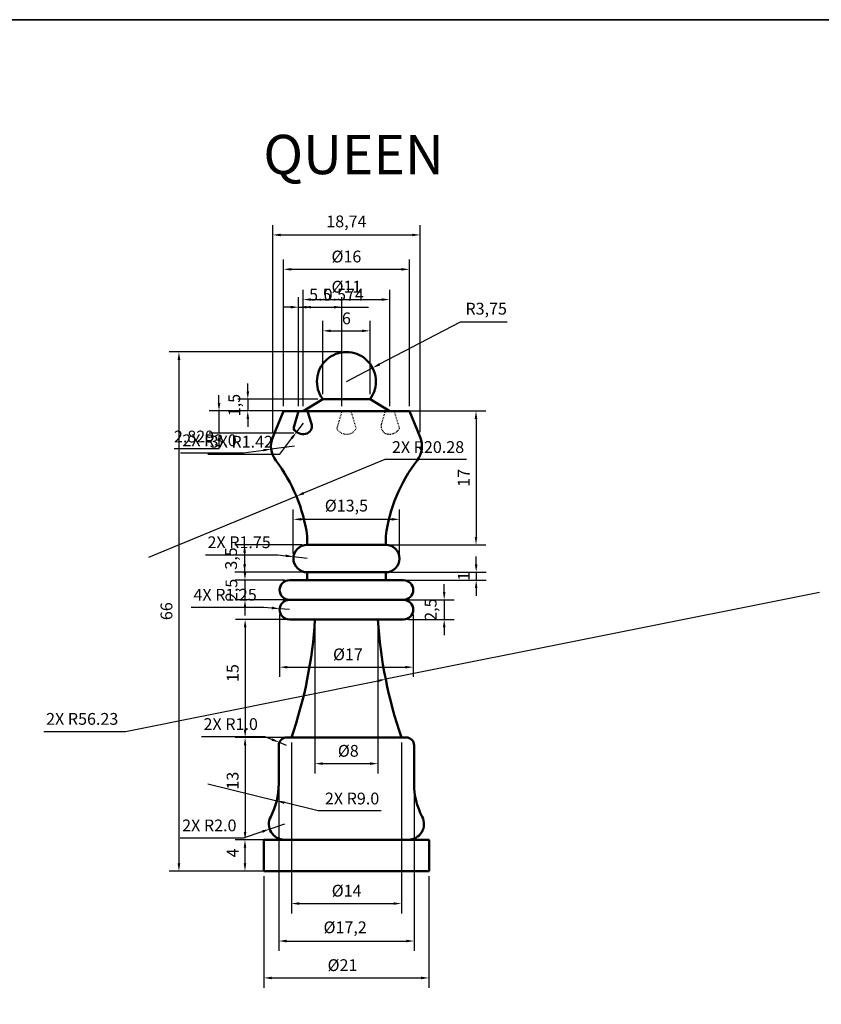
# Model space of a CAD drawing. Units: millimetres. Extents: x 172 to 469, y -14 to 196.
# Tile 4 of 5: x 279 to 381, y 71 to 196. Entities that reach past the tile are written whole.
import ezdxf

# ---------------------------------------------------------------- set-up
doc = ezdxf.new("R2010")
doc.units = ezdxf.units.MM
doc.header["$LTSCALE"] = 0.1
doc.linetypes.add('HIDDEN', pattern=[9.525, 6.35, -3.175])
for name, color, linetype, lineweight in [('M-DIMS', 2, 'Continuous', 25), ('M-HIDN', 1, 'HIDDEN', 25), ('M-OUTL', 7, 'Continuous', 50), ('M-TEXT', 3, 'Continuous', 25), ('M-TTLB', 7, 'Continuous', 35)]:
    doc.layers.add(name, color=color, linetype=linetype, lineweight=lineweight)
doc.styles.get("Standard").update_dxf_attribs({"font": 'arial.ttf'})
doc.dimstyles.new('ISO-25', dxfattribs={"dimtxt": 1.5, "dimasz": 1, "dimexe": 1.25, "dimexo": 0.625, "dimtad": 1, "dimtoh": 1, "dimtxsty": 'Standard', "dimcen": 2.5, "dimadec": 0, "dimazin": 0, "dimtfac": 1, "dimtmove": 0, "dimatfit": 3, "dimfxl": 1, "dimarcsym": 0})

# ---------------------------------------------------------------- blocks, each defined once
blk = doc.blocks.new('*D15')
at = {"layer": 'Defpoints', "color": 0, "ltscale": 0.1, "transparency": 16777216}
for p in [(328.72, 164.14), (312.72, 146.13), (328.72, 146.13)]:
    blk.add_point(p, dxfattribs=at)
at = {"layer": 'M-DIMS', "color": 0, "lineweight": -2, "ltscale": 0.1, "transparency": 16777216}
for p, q in [((312.72, 146.75), (312.72, 165.39)), ((328.72, 146.75), (328.72, 165.39)), ((313.72, 164.14), (327.72, 164.14))]:
    blk.add_line(p, q, dxfattribs=at)
at = {"layer": 'M-DIMS', "color": 0, "ltscale": 0.1, "transparency": 16777216}
for points in [[(313.72, 164.3), (313.72, 163.97), (312.72, 164.14)], [(327.72, 164.3), (327.72, 163.97), (328.72, 164.14)]]:
    blk.add_solid(points, dxfattribs=at)
at = {"layer": 'M-DIMS', "color": 0, "ltscale": 0.1, "transparency": 16777216, "insert": (320.72, 165.57), "char_height": 1.5, "attachment_point": 5}
blk.add_mtext('%%C16', dxfattribs=at)
blk = doc.blocks.new('*D16')
at = {"layer": 'Defpoints', "color": 0, "ltscale": 0.1, "transparency": 16777216}
for p in [(330.1, 168.51), (311.35, 142.82), (330.1, 142.82)]:
    blk.add_point(p, dxfattribs=at)
at = {"layer": 'M-DIMS', "color": 0, "lineweight": -2, "ltscale": 0.1, "transparency": 16777216}
for p, q in [((311.35, 143.44), (311.35, 169.76)), ((330.1, 143.44), (330.1, 169.76)), ((312.35, 168.51), (329.1, 168.51))]:
    blk.add_line(p, q, dxfattribs=at)
at = {"layer": 'M-DIMS', "color": 0, "ltscale": 0.1, "transparency": 16777216}
for points in [[(312.35, 168.67), (312.35, 168.34), (311.35, 168.51)], [(329.1, 168.67), (329.1, 168.34), (330.1, 168.51)]]:
    blk.add_solid(points, dxfattribs=at)
at = {"layer": 'M-DIMS', "color": 0, "ltscale": 0.1, "transparency": 16777216, "insert": (320.72, 170.03), "char_height": 1.5, "attachment_point": 5}
blk.add_mtext('18,74', dxfattribs=at)
blk = doc.blocks.new('*D17')
at = {"layer": 'Defpoints', "color": 0, "ltscale": 0.1, "transparency": 16777216}
for p in [(326.22, 160.29), (315.22, 146.13), (326.22, 146.13)]:
    blk.add_point(p, dxfattribs=at)
at = {"layer": 'M-DIMS', "color": 0, "lineweight": -2, "ltscale": 0.1, "transparency": 16777216}
for p, q in [((315.22, 146.75), (315.22, 161.54)), ((326.22, 146.75), (326.22, 161.54)), ((316.22, 160.29), (325.22, 160.29))]:
    blk.add_line(p, q, dxfattribs=at)
at = {"layer": 'M-DIMS', "color": 0, "ltscale": 0.1, "transparency": 16777216}
for points in [[(316.22, 160.46), (316.22, 160.13), (315.22, 160.29)], [(325.22, 160.46), (325.22, 160.13), (326.22, 160.29)]]:
    blk.add_solid(points, dxfattribs=at)
at = {"layer": 'M-DIMS', "color": 0, "ltscale": 0.1, "transparency": 16777216, "insert": (320.72, 161.73), "char_height": 1.5, "attachment_point": 5}
blk.add_mtext('%%C11', dxfattribs=at)
blk = doc.blocks.new('*D18')
at = {"layer": 'Defpoints', "color": 0, "ltscale": 0.1, "transparency": 16777216}
for p in [(323.72, 156.32), (317.72, 147.63), (323.72, 147.63)]:
    blk.add_point(p, dxfattribs=at)
at = {"layer": 'M-DIMS', "color": 0, "lineweight": -2, "ltscale": 0.1, "transparency": 16777216}
for p, q in [((317.72, 148.25), (317.72, 157.57)), ((323.72, 148.25), (323.72, 157.57)), ((318.72, 156.32), (322.72, 156.32))]:
    blk.add_line(p, q, dxfattribs=at)
at = {"layer": 'M-DIMS', "color": 0, "ltscale": 0.1, "transparency": 16777216}
for points in [[(318.72, 156.48), (318.72, 156.15), (317.72, 156.32)], [(322.72, 156.48), (322.72, 156.15), (323.72, 156.32)]]:
    blk.add_solid(points, dxfattribs=at)
at = {"layer": 'M-DIMS', "color": 0, "ltscale": 0.1, "transparency": 16777216, "insert": (320.72, 157.71), "char_height": 1.5, "attachment_point": 5}
blk.add_mtext('6', dxfattribs=at)
blk = doc.blocks.new('*D19')
at = {"layer": 'Defpoints', "color": 0, "ltscale": 0.1, "transparency": 16777216}
for p in [(324.05, 151.61), (320.72, 149.88)]:
    blk.add_point(p, dxfattribs=at)
at = {"layer": 'M-DIMS', "color": 0, "lineweight": -2, "ltscale": 0.1, "transparency": 16777216}
for p, q in [((335.19, 157.41), (324.94, 152.07)), ((341.16, 157.41), (335.19, 157.41)), ((320.72, 149.88), (324.05, 151.61))]:
    blk.add_line(p, q, dxfattribs=at)
at = {"layer": 'M-DIMS', "color": 0, "ltscale": 0.1, "transparency": 16777216}
blk.add_solid([(324.86, 152.22), (325.01, 151.92), (324.05, 151.61)], dxfattribs=at)
at = {"layer": 'M-DIMS', "color": 0, "ltscale": 0.1, "transparency": 16777216, "insert": (338.49, 158.94), "char_height": 1.5, "attachment_point": 5}
blk.add_mtext('R3,75', dxfattribs=at)
blk = doc.blocks.new('*D20')
at = {"layer": 'Defpoints', "color": 0, "ltscale": 0.1, "transparency": 16777216}
for p in [(327.72, 146.13), (324.58, 129.13), (337.2, 129.13)]:
    blk.add_point(p, dxfattribs=at)
at = {"layer": 'M-DIMS', "color": 0, "lineweight": -2, "ltscale": 0.1, "transparency": 16777216}
for p, q in [((328.34, 146.13), (338.45, 146.13)), ((337.2, 145.13), (337.2, 130.13)), ((325.2, 129.13), (338.45, 129.13))]:
    blk.add_line(p, q, dxfattribs=at)
at = {"layer": 'M-DIMS', "color": 0, "ltscale": 0.1, "transparency": 16777216}
for points in [[(337.03, 145.13), (337.36, 145.13), (337.2, 146.13)], [(337.03, 130.13), (337.36, 130.13), (337.2, 129.13)]]:
    blk.add_solid(points, dxfattribs=at)
at = {"layer": 'M-DIMS', "color": 0, "ltscale": 0.1, "transparency": 16777216, "insert": (335.82, 137.63), "char_height": 1.5, "attachment_point": 5, "rotation": 90}
blk.add_mtext('17', dxfattribs=at)
blk = doc.blocks.new('*D21')
at = {"layer": 'Defpoints', "color": 0, "ltscale": 0.1, "transparency": 16777216}
for p in [(327.47, 132.36), (313.97, 127.38), (327.47, 127.38)]:
    blk.add_point(p, dxfattribs=at)
at = {"layer": 'M-DIMS', "color": 0, "lineweight": -2, "ltscale": 0.1, "transparency": 16777216}
for p, q in [((313.97, 128), (313.97, 133.61)), ((327.47, 128), (327.47, 133.61)), ((314.97, 132.36), (326.47, 132.36))]:
    blk.add_line(p, q, dxfattribs=at)
at = {"layer": 'M-DIMS', "color": 0, "ltscale": 0.1, "transparency": 16777216}
for points in [[(314.97, 132.53), (314.97, 132.2), (313.97, 132.36)], [(326.47, 132.53), (326.47, 132.2), (327.47, 132.36)]]:
    blk.add_solid(points, dxfattribs=at)
at = {"layer": 'M-DIMS', "color": 0, "ltscale": 0.1, "transparency": 16777216, "insert": (320.72, 133.91), "char_height": 1.5, "attachment_point": 5}
blk.add_mtext('%%C13,5', dxfattribs=at)
blk = doc.blocks.new('*D22')
at = {"layer": 'Defpoints', "color": 0, "ltscale": 0.1, "transparency": 16777216}
for p in [(315.72, 129.13), (307.78, 125.63), (315.72, 125.63)]:
    blk.add_point(p, dxfattribs=at)
at = {"layer": 'M-DIMS', "color": 0, "lineweight": -2, "ltscale": 0.1, "transparency": 16777216}
for p, q in [((315.1, 129.13), (306.53, 129.13)), ((307.78, 128.13), (307.78, 126.63)), ((315.1, 125.63), (306.53, 125.63))]:
    blk.add_line(p, q, dxfattribs=at)
at = {"layer": 'M-DIMS', "color": 0, "ltscale": 0.1, "transparency": 16777216}
for points in [[(307.61, 128.13), (307.95, 128.13), (307.78, 129.13)], [(307.61, 126.63), (307.95, 126.63), (307.78, 125.63)]]:
    blk.add_solid(points, dxfattribs=at)
at = {"layer": 'M-DIMS', "color": 0, "ltscale": 0.1, "transparency": 16777216, "insert": (306.25, 127.38), "char_height": 1.5, "attachment_point": 5, "rotation": 90}
blk.add_mtext('3,5', dxfattribs=at)
blk = doc.blocks.new('*D23')
at = {"layer": 'Defpoints', "color": 0, "ltscale": 0.1, "transparency": 16777216}
for p in [(317.72, 147.63), (308.18, 146.13), (317.72, 146.13)]:
    blk.add_point(p, dxfattribs=at)
at = {"layer": 'M-DIMS', "color": 0, "lineweight": -2, "ltscale": 0.1, "transparency": 16777216}
for p, q in [((308.18, 148.63), (308.18, 149.63)), ((317.1, 147.63), (306.93, 147.63)), ((308.18, 147.63), (308.18, 146.13)), ((317.1, 146.13), (306.93, 146.13)), ((308.18, 145.13), (308.18, 144.13))]:
    blk.add_line(p, q, dxfattribs=at)
at = {"layer": 'M-DIMS', "color": 0, "ltscale": 0.1, "transparency": 16777216}
for points in [[(308.02, 148.63), (308.35, 148.63), (308.18, 147.63)], [(308.02, 145.13), (308.35, 145.13), (308.18, 146.13)]]:
    blk.add_solid(points, dxfattribs=at)
at = {"layer": 'M-DIMS', "color": 0, "ltscale": 0.1, "transparency": 16777216, "insert": (306.66, 146.88), "char_height": 1.5, "attachment_point": 5, "rotation": 90}
blk.add_mtext('1,5', dxfattribs=at)
blk = doc.blocks.new('*D24')
at = {"layer": 'Defpoints', "color": 0, "ltscale": 0.1, "transparency": 16777216}
for p in [(325.72, 125.63), (325.72, 124.63), (337.22, 124.63)]:
    blk.add_point(p, dxfattribs=at)
at = {"layer": 'M-DIMS', "color": 0, "lineweight": -2, "ltscale": 0.1, "transparency": 16777216}
for p, q in [((337.22, 126.63), (337.22, 127.63)), ((326.35, 125.63), (338.47, 125.63)), ((337.22, 125.63), (337.22, 124.63)), ((326.35, 124.63), (338.47, 124.63)), ((337.22, 123.63), (337.22, 122.63))]:
    blk.add_line(p, q, dxfattribs=at)
at = {"layer": 'M-DIMS', "color": 0, "ltscale": 0.1, "transparency": 16777216}
for points in [[(337.05, 126.63), (337.38, 126.63), (337.22, 125.63)], [(337.05, 123.63), (337.38, 123.63), (337.22, 124.63)]]:
    blk.add_solid(points, dxfattribs=at)
at = {"layer": 'M-DIMS', "color": 0, "ltscale": 0.1, "transparency": 16777216, "insert": (335.84, 125.13), "char_height": 1.5, "attachment_point": 5, "rotation": 90}
blk.add_mtext('1', dxfattribs=at)
blk = doc.blocks.new('*D25')
at = {"layer": 'Defpoints', "color": 0, "ltscale": 0.1, "transparency": 16777216}
for p in [(313.47, 124.63), (307.82, 122.13), (313.47, 122.13)]:
    blk.add_point(p, dxfattribs=at)
at = {"layer": 'M-DIMS', "color": 0, "lineweight": -2, "ltscale": 0.1, "transparency": 16777216}
for p, q in [((307.82, 125.63), (307.82, 126.63)), ((312.85, 124.63), (306.57, 124.63)), ((307.82, 124.63), (307.82, 122.13)), ((312.85, 122.13), (306.57, 122.13)), ((307.82, 121.13), (307.82, 120.13))]:
    blk.add_line(p, q, dxfattribs=at)
at = {"layer": 'M-DIMS', "color": 0, "ltscale": 0.1, "transparency": 16777216}
for points in [[(307.66, 125.63), (307.99, 125.63), (307.82, 124.63)], [(307.66, 121.13), (307.99, 121.13), (307.82, 122.13)]]:
    blk.add_solid(points, dxfattribs=at)
at = {"layer": 'M-DIMS', "color": 0, "ltscale": 0.1, "transparency": 16777216, "insert": (306.3, 123.38), "char_height": 1.5, "attachment_point": 5, "rotation": 90}
blk.add_mtext('2,5', dxfattribs=at)
blk = doc.blocks.new('*D26')
at = {"layer": 'Defpoints', "color": 0, "ltscale": 0.1, "transparency": 16777216}
for p in [(327.97, 122.13), (327.97, 119.63), (333.15, 119.63)]:
    blk.add_point(p, dxfattribs=at)
at = {"layer": 'M-DIMS', "color": 0, "lineweight": -2, "ltscale": 0.1, "transparency": 16777216}
for p, q in [((333.15, 123.13), (333.15, 124.13)), ((328.6, 122.13), (334.4, 122.13)), ((333.15, 122.13), (333.15, 119.63)), ((328.6, 119.63), (334.4, 119.63)), ((333.15, 118.63), (333.15, 117.63))]:
    blk.add_line(p, q, dxfattribs=at)
at = {"layer": 'M-DIMS', "color": 0, "ltscale": 0.1, "transparency": 16777216}
for points in [[(332.99, 123.13), (333.32, 123.13), (333.15, 122.13)], [(332.99, 118.63), (333.32, 118.63), (333.15, 119.63)]]:
    blk.add_solid(points, dxfattribs=at)
at = {"layer": 'M-DIMS', "color": 0, "ltscale": 0.1, "transparency": 16777216, "insert": (331.63, 120.88), "char_height": 1.5, "attachment_point": 5, "rotation": 90}
blk.add_mtext('2,5', dxfattribs=at)
blk = doc.blocks.new('*D27')
at = {"layer": 'Defpoints', "color": 0, "ltscale": 0.1, "transparency": 16777216}
for p in [(320.72, 119.63), (307.85, 104.63), (320.72, 104.63)]:
    blk.add_point(p, dxfattribs=at)
at = {"layer": 'M-DIMS', "color": 0, "lineweight": -2, "ltscale": 0.1, "transparency": 16777216}
for p, q in [((320.1, 119.63), (306.6, 119.63)), ((307.85, 118.63), (307.85, 105.63)), ((320.1, 104.63), (306.6, 104.63))]:
    blk.add_line(p, q, dxfattribs=at)
at = {"layer": 'M-DIMS', "color": 0, "ltscale": 0.1, "transparency": 16777216}
for points in [[(307.68, 118.63), (308.01, 118.63), (307.85, 119.63)], [(307.68, 105.63), (308.01, 105.63), (307.85, 104.63)]]:
    blk.add_solid(points, dxfattribs=at)
at = {"layer": 'M-DIMS', "color": 0, "ltscale": 0.1, "transparency": 16777216, "insert": (306.46, 112.82), "char_height": 1.5, "attachment_point": 5, "rotation": 90}
blk.add_mtext('15', dxfattribs=at)
blk = doc.blocks.new('*D28')
at = {"layer": 'Defpoints', "color": 0, "ltscale": 0.1, "transparency": 16777216}
for p in [(312.22, 120.88), (329.22, 120.88), (329.22, 113.57)]:
    blk.add_point(p, dxfattribs=at)
at = {"layer": 'M-DIMS', "color": 0, "lineweight": -2, "ltscale": 0.1, "transparency": 16777216}
for p, q in [((312.22, 120.25), (312.22, 112.32)), ((329.22, 120.25), (329.22, 112.32)), ((313.22, 113.57), (328.22, 113.57))]:
    blk.add_line(p, q, dxfattribs=at)
at = {"layer": 'M-DIMS', "color": 0, "ltscale": 0.1, "transparency": 16777216}
for points in [[(313.22, 113.73), (313.22, 113.4), (312.22, 113.57)], [(328.22, 113.73), (328.22, 113.4), (329.22, 113.57)]]:
    blk.add_solid(points, dxfattribs=at)
at = {"layer": 'M-DIMS', "color": 0, "ltscale": 0.1, "transparency": 16777216, "insert": (320.91, 115), "char_height": 1.5, "attachment_point": 5}
blk.add_mtext('%%C17', dxfattribs=at)
blk = doc.blocks.new('*D29')
at = {"layer": 'Defpoints', "color": 0, "ltscale": 0.1, "transparency": 16777216}
for p in [(316.72, 119.63), (324.72, 119.63), (324.72, 101.31)]:
    blk.add_point(p, dxfattribs=at)
at = {"layer": 'M-DIMS', "color": 0, "lineweight": -2, "ltscale": 0.1, "transparency": 16777216}
for p, q in [((316.72, 119), (316.72, 100.06)), ((324.72, 119), (324.72, 100.06)), ((317.72, 101.31), (323.72, 101.31))]:
    blk.add_line(p, q, dxfattribs=at)
at = {"layer": 'M-DIMS', "color": 0, "ltscale": 0.1, "transparency": 16777216}
for points in [[(317.72, 101.48), (317.72, 101.14), (316.72, 101.31)], [(323.72, 101.48), (323.72, 101.14), (324.72, 101.31)]]:
    blk.add_solid(points, dxfattribs=at)
at = {"layer": 'M-DIMS', "color": 0, "ltscale": 0.1, "transparency": 16777216, "insert": (320.96, 102.74), "char_height": 1.5, "attachment_point": 5}
blk.add_mtext('%%C8', dxfattribs=at)
blk = doc.blocks.new('*D30')
at = {"layer": 'Defpoints', "color": 0, "ltscale": 0.1, "transparency": 16777216}
for p in [(313.72, 104.63), (327.72, 104.63), (327.72, 83.52)]:
    blk.add_point(p, dxfattribs=at)
at = {"layer": 'M-DIMS', "color": 0, "lineweight": -2, "ltscale": 0.1, "transparency": 16777216}
for p, q in [((313.72, 104), (313.72, 82.27)), ((327.72, 104), (327.72, 82.27)), ((314.72, 83.52), (326.72, 83.52))]:
    blk.add_line(p, q, dxfattribs=at)
at = {"layer": 'M-DIMS', "color": 0, "ltscale": 0.1, "transparency": 16777216}
for points in [[(314.72, 83.69), (314.72, 83.36), (313.72, 83.52)], [(326.72, 83.69), (326.72, 83.36), (327.72, 83.52)]]:
    blk.add_solid(points, dxfattribs=at)
at = {"layer": 'M-DIMS', "color": 0, "ltscale": 0.1, "transparency": 16777216, "insert": (320.75, 84.96), "char_height": 1.5, "attachment_point": 5}
blk.add_mtext('%%C14', dxfattribs=at)
blk = doc.blocks.new('*D31')
at = {"layer": 'Defpoints', "color": 0, "ltscale": 0.1, "transparency": 16777216}
for p in [(312.12, 101.18), (329.32, 101.18), (329.32, 78.76)]:
    blk.add_point(p, dxfattribs=at)
at = {"layer": 'M-DIMS', "color": 0, "lineweight": -2, "ltscale": 0.1, "transparency": 16777216}
for p, q in [((312.12, 100.56), (312.12, 77.51)), ((329.32, 100.56), (329.32, 77.51)), ((313.12, 78.76), (328.32, 78.76))]:
    blk.add_line(p, q, dxfattribs=at)
at = {"layer": 'M-DIMS', "color": 0, "ltscale": 0.1, "transparency": 16777216}
for points in [[(313.12, 78.93), (313.12, 78.59), (312.12, 78.76)], [(328.32, 78.93), (328.32, 78.59), (329.32, 78.76)]]:
    blk.add_solid(points, dxfattribs=at)
at = {"layer": 'M-DIMS', "color": 0, "ltscale": 0.1, "transparency": 16777216, "insert": (320.56, 80.31), "char_height": 1.5, "attachment_point": 5}
blk.add_mtext('%%C17,2', dxfattribs=at)
blk = doc.blocks.new('*D32')
at = {"layer": 'Defpoints', "color": 0, "ltscale": 0.1, "transparency": 16777216}
for p in [(310.22, 87.63), (331.22, 87.63), (331.22, 74.07)]:
    blk.add_point(p, dxfattribs=at)
at = {"layer": 'M-DIMS', "color": 0, "lineweight": -2, "ltscale": 0.1, "transparency": 16777216}
for p, q in [((310.22, 87), (310.22, 72.82)), ((331.22, 87), (331.22, 72.82)), ((311.22, 74.07), (330.22, 74.07))]:
    blk.add_line(p, q, dxfattribs=at)
at = {"layer": 'M-DIMS', "color": 0, "ltscale": 0.1, "transparency": 16777216}
for points in [[(311.22, 74.23), (311.22, 73.9), (310.22, 74.07)], [(330.22, 74.23), (330.22, 73.9), (331.22, 74.07)]]:
    blk.add_solid(points, dxfattribs=at)
at = {"layer": 'M-DIMS', "color": 0, "ltscale": 0.1, "transparency": 16777216, "insert": (320.22, 75.5), "char_height": 1.5, "attachment_point": 5}
blk.add_mtext('%%C21', dxfattribs=at)
blk = doc.blocks.new('*D33')
at = {"layer": 'Defpoints', "color": 0, "ltscale": 0.1, "transparency": 16777216}
for p in [(320.72, 153.63), (299.43, 87.63), (320.72, 87.63)]:
    blk.add_point(p, dxfattribs=at)
at = {"layer": 'M-DIMS', "color": 0, "lineweight": -2, "ltscale": 0.1, "transparency": 16777216}
for p, q in [((320.1, 153.63), (298.18, 153.63)), ((299.43, 152.63), (299.43, 88.63)), ((320.1, 87.63), (298.18, 87.63))]:
    blk.add_line(p, q, dxfattribs=at)
at = {"layer": 'M-DIMS', "color": 0, "ltscale": 0.1, "transparency": 16777216}
for points in [[(299.26, 152.63), (299.6, 152.63), (299.43, 153.63)], [(299.26, 88.63), (299.6, 88.63), (299.43, 87.63)]]:
    blk.add_solid(points, dxfattribs=at)
at = {"layer": 'M-DIMS', "color": 0, "ltscale": 0.1, "transparency": 16777216, "insert": (298.04, 120.68), "char_height": 1.5, "attachment_point": 5, "rotation": 90}
blk.add_mtext('66', dxfattribs=at)
blk = doc.blocks.new('*D34')
at = {"layer": 'Defpoints', "color": 0, "ltscale": 0.1, "transparency": 16777216}
for p in [(313.72, 104.63), (307.84, 91.63), (313.72, 91.63)]:
    blk.add_point(p, dxfattribs=at)
at = {"layer": 'M-DIMS', "color": 0, "lineweight": -2, "ltscale": 0.1, "transparency": 16777216}
for p, q in [((313.1, 104.63), (306.59, 104.63)), ((307.84, 103.63), (307.84, 92.63)), ((313.1, 91.63), (306.59, 91.63))]:
    blk.add_line(p, q, dxfattribs=at)
at = {"layer": 'M-DIMS', "color": 0, "ltscale": 0.1, "transparency": 16777216}
for points in [[(307.67, 103.63), (308, 103.63), (307.84, 104.63)], [(307.67, 92.63), (308, 92.63), (307.84, 91.63)]]:
    blk.add_solid(points, dxfattribs=at)
at = {"layer": 'M-DIMS', "color": 0, "ltscale": 0.1, "transparency": 16777216, "insert": (306.45, 99.14), "char_height": 1.5, "attachment_point": 5, "rotation": 90}
blk.add_mtext('13', dxfattribs=at)
blk = doc.blocks.new('*D35')
at = {"layer": 'Defpoints', "color": 0, "ltscale": 0.1, "transparency": 16777216}
for p in [(310.22, 91.63), (307.82, 87.63), (310.22, 87.63)]:
    blk.add_point(p, dxfattribs=at)
at = {"layer": 'M-DIMS', "color": 0, "lineweight": -2, "ltscale": 0.1, "transparency": 16777216}
for p, q in [((309.6, 91.63), (306.57, 91.63)), ((307.82, 90.63), (307.82, 88.63)), ((309.6, 87.63), (306.57, 87.63))]:
    blk.add_line(p, q, dxfattribs=at)
at = {"layer": 'M-DIMS', "color": 0, "ltscale": 0.1, "transparency": 16777216}
for points in [[(307.66, 90.63), (307.99, 90.63), (307.82, 91.63)], [(307.66, 88.63), (307.99, 88.63), (307.82, 87.63)]]:
    blk.add_solid(points, dxfattribs=at)
at = {"layer": 'M-DIMS', "color": 0, "ltscale": 0.1, "transparency": 16777216, "insert": (306.45, 89.96), "char_height": 1.5, "attachment_point": 5, "rotation": 90}
blk.add_mtext('4', dxfattribs=at)
blk = doc.blocks.new('*D61')
at = {"layer": 'Defpoints', "color": 0, "ltscale": 0.1, "transparency": 16777216}
for p in [(315.22, 159.33), (314.65, 146.13), (315.22, 146.13)]:
    blk.add_point(p, dxfattribs=at)
at = {"layer": 'M-DIMS', "color": 0, "lineweight": -2, "ltscale": 0.1, "transparency": 16777216}
for p, q in [((314.65, 146.75), (314.65, 160.58)), ((315.22, 146.75), (315.22, 160.58)), ((313.65, 159.33), (312.65, 159.33)), ((314.65, 159.33), (315.22, 159.33)), ((316.22, 159.33), (323.53, 159.33))]:
    blk.add_line(p, q, dxfattribs=at)
at = {"layer": 'M-DIMS', "color": 0, "ltscale": 0.1, "transparency": 16777216}
for points in [[(313.65, 159.49), (313.65, 159.16), (314.65, 159.33)], [(316.22, 159.49), (316.22, 159.16), (315.22, 159.33)]]:
    blk.add_solid(points, dxfattribs=at)
at = {"layer": 'M-DIMS', "color": 0, "ltscale": 0.1, "transparency": 16777216, "insert": (320.38, 160.72), "char_height": 1.5, "attachment_point": 5}
blk.add_mtext('0.574', dxfattribs=at)
blk = doc.blocks.new('*D62')
at = {"layer": 'Defpoints', "color": 0, "ltscale": 0.1, "transparency": 16777216}
for p in [(320.15, 159.33), (314.65, 146.13), (320.15, 146.13)]:
    blk.add_point(p, dxfattribs=at)
at = {"layer": 'M-DIMS', "color": 0, "lineweight": -2, "ltscale": 0.1, "transparency": 16777216}
for p, q in [((314.65, 146.75), (314.65, 160.58)), ((320.15, 146.75), (320.15, 160.58)), ((315.65, 159.33), (319.15, 159.33))]:
    blk.add_line(p, q, dxfattribs=at)
at = {"layer": 'M-DIMS', "color": 0, "ltscale": 0.1, "transparency": 16777216}
for points in [[(315.65, 159.49), (315.65, 159.16), (314.65, 159.33)], [(319.15, 159.49), (319.15, 159.16), (320.15, 159.33)]]:
    blk.add_solid(points, dxfattribs=at)
at = {"layer": 'M-DIMS', "color": 0, "ltscale": 0.1, "transparency": 16777216, "insert": (317.4, 160.72), "char_height": 1.5, "attachment_point": 5}
blk.add_mtext('5.5', dxfattribs=at)
blk = doc.blocks.new('*D63')
at = {"layer": 'Defpoints', "color": 0, "ltscale": 0.1, "transparency": 16777216}
for p in [(314.65, 146.13), (304.52, 143.3), (314.66, 143.3)]:
    blk.add_point(p, dxfattribs=at)
at = {"layer": 'M-DIMS', "color": 0, "lineweight": -2, "ltscale": 0.1, "transparency": 16777216}
for p, q in [((304.52, 147.13), (304.52, 148.13)), ((314.02, 146.13), (303.27, 146.13)), ((304.52, 146.13), (304.52, 143.3)), ((314.03, 143.3), (303.27, 143.3)), ((304.52, 142.3), (304.52, 141.3)), ((304.52, 141.3), (298.81, 141.3))]:
    blk.add_line(p, q, dxfattribs=at)
at = {"layer": 'M-DIMS', "color": 0, "ltscale": 0.1, "transparency": 16777216}
for points in [[(304.36, 147.13), (304.69, 147.13), (304.52, 146.13)], [(304.36, 142.3), (304.69, 142.3), (304.52, 143.3)]]:
    blk.add_solid(points, dxfattribs=at)
at = {"layer": 'M-DIMS', "color": 0, "ltscale": 0.1, "transparency": 16777216, "insert": (301.35, 142.69), "char_height": 1.5, "attachment_point": 5}
blk.add_mtext('2.829', dxfattribs=at)
blk = doc.blocks.new('*D74')
at = {"layer": 'Defpoints', "color": 0, "ltscale": 0.1, "transparency": 16777216}
for p in [(380.85, 123.05), (325.71, 112.03)]:
    blk.add_point(p, dxfattribs=at)
at = {"layer": 'M-DIMS', "color": 0, "lineweight": -2, "ltscale": 0.1, "transparency": 16777216}
for p, q in [((380.85, 123.05), (325.71, 112.03)), ((292.63, 105.41), (324.73, 111.83)), ((282.26, 105.41), (292.63, 105.41))]:
    blk.add_line(p, q, dxfattribs=at)
at = {"layer": 'M-DIMS', "color": 0, "ltscale": 0.1, "transparency": 16777216}
blk.add_solid([(324.7, 111.99), (324.76, 111.67), (325.71, 112.03)], dxfattribs=at)
at = {"layer": 'M-DIMS', "color": 0, "ltscale": 0.1, "transparency": 16777216, "insert": (287.13, 106.8), "char_height": 1.5, "attachment_point": 5}
blk.add_mtext('2X R56.23', dxfattribs=at)
blk = doc.blocks.new('*D75')
at = {"layer": 'Defpoints', "color": 0, "ltscale": 0.1, "transparency": 16777216}
for p in [(314.36, 135.3), (295.62, 127.53)]:
    blk.add_point(p, dxfattribs=at)
at = {"layer": 'M-DIMS', "color": 0, "lineweight": -2, "ltscale": 0.1, "transparency": 16777216}
for p, q in [((325.6, 139.96), (315.28, 135.69)), ((335.97, 139.96), (325.6, 139.96)), ((295.62, 127.53), (314.36, 135.3))]:
    blk.add_line(p, q, dxfattribs=at)
at = {"layer": 'M-DIMS', "color": 0, "ltscale": 0.1, "transparency": 16777216}
blk.add_solid([(315.22, 135.84), (315.35, 135.53), (314.36, 135.3)], dxfattribs=at)
at = {"layer": 'M-DIMS', "color": 0, "ltscale": 0.1, "transparency": 16777216, "insert": (331.1, 141.35), "char_height": 1.5, "attachment_point": 5}
blk.add_mtext('2X R20.28', dxfattribs=at)
blk = doc.blocks.new('*D76')
at = {"layer": 'Defpoints', "color": 0, "ltscale": 0.1, "transparency": 16777216}
for p in [(303.12, 98.74), (311.86, 96.59)]:
    blk.add_point(p, dxfattribs=at)
at = {"layer": 'M-DIMS', "color": 0, "lineweight": -2, "ltscale": 0.1, "transparency": 16777216}
for p, q in [((303.12, 98.74), (311.86, 96.59)), ((317.11, 95.29), (312.83, 96.35)), ((325.14, 95.29), (317.11, 95.29))]:
    blk.add_line(p, q, dxfattribs=at)
at = {"layer": 'M-DIMS', "color": 0, "ltscale": 0.1, "transparency": 16777216}
blk.add_solid([(312.87, 96.51), (312.79, 96.18), (311.86, 96.59)], dxfattribs=at)
at = {"layer": 'M-DIMS', "color": 0, "ltscale": 0.1, "transparency": 16777216, "insert": (321.44, 96.68), "char_height": 1.5, "attachment_point": 5}
blk.add_mtext('2X R9.0', dxfattribs=at)
blk = doc.blocks.new('*D77')
at = {"layer": 'Defpoints', "color": 0, "ltscale": 0.1, "transparency": 16777216}
for p in [(314.12, 141.67), (311.15, 141.28)]:
    blk.add_point(p, dxfattribs=at)
at = {"layer": 'M-DIMS', "color": 0, "lineweight": -2, "ltscale": 0.1, "transparency": 16777216}
for p, q in [((314.12, 141.67), (311.15, 141.28)), ((299.61, 140.82), (307.65, 140.82)), ((307.65, 140.82), (310.16, 141.15))]:
    blk.add_line(p, q, dxfattribs=at)
at = {"layer": 'M-DIMS', "color": 0, "ltscale": 0.1, "transparency": 16777216}
blk.add_solid([(310.14, 141.32), (310.18, 140.99), (311.15, 141.28)], dxfattribs=at)
at = {"layer": 'M-DIMS', "color": 0, "ltscale": 0.1, "transparency": 16777216, "insert": (303.32, 142.21), "char_height": 1.5, "attachment_point": 5}
blk.add_mtext('2X R3.0', dxfattribs=at)
blk = doc.blocks.new('*D78')
at = {"layer": 'Defpoints', "color": 0, "ltscale": 0.1, "transparency": 16777216}
for p in [(310.97, 92.99), (312.87, 93.63)]:
    blk.add_point(p, dxfattribs=at)
at = {"layer": 'M-DIMS', "color": 0, "lineweight": -2, "ltscale": 0.1, "transparency": 16777216}
for p, q in [((307.62, 91.87), (310.02, 92.67)), ((312.87, 93.63), (310.97, 92.99)), ((299.59, 91.87), (307.62, 91.87))]:
    blk.add_line(p, q, dxfattribs=at)
at = {"layer": 'M-DIMS', "color": 0, "ltscale": 0.1, "transparency": 16777216}
blk.add_solid([(309.97, 92.83), (310.07, 92.51), (310.97, 92.99)], dxfattribs=at)
at = {"layer": 'M-DIMS', "color": 0, "ltscale": 0.1, "transparency": 16777216, "insert": (303.29, 93.26), "char_height": 1.5, "attachment_point": 5}
blk.add_mtext('2X R2.0', dxfattribs=at)
blk = doc.blocks.new('*D79')
at = {"layer": 'Defpoints', "color": 0, "ltscale": 0.1, "transparency": 16777216}
for p in [(312.2, 104), (313.12, 103.63)]:
    blk.add_point(p, dxfattribs=at)
at = {"layer": 'M-DIMS', "color": 0, "lineweight": -2, "ltscale": 0.1, "transparency": 16777216}
for p, q in [((302.3, 104.75), (310.34, 104.75)), ((310.34, 104.75), (311.27, 104.37)), ((313.12, 103.63), (312.2, 104))]:
    blk.add_line(p, q, dxfattribs=at)
at = {"layer": 'M-DIMS', "color": 0, "ltscale": 0.1, "transparency": 16777216}
blk.add_solid([(311.33, 104.53), (311.21, 104.22), (312.2, 104)], dxfattribs=at)
at = {"layer": 'M-DIMS', "color": 0, "ltscale": 0.1, "transparency": 16777216, "insert": (306.01, 106.14), "char_height": 1.5, "attachment_point": 5}
blk.add_mtext('2X R1.0', dxfattribs=at)
blk = doc.blocks.new('*D80')
at = {"layer": 'Defpoints', "color": 0, "ltscale": 0.1, "transparency": 16777216}
for p in [(315.22, 144.6), (314.37, 143.46)]:
    blk.add_point(p, dxfattribs=at)
at = {"layer": 'M-DIMS', "color": 0, "lineweight": -2, "ltscale": 0.1, "transparency": 16777216}
for p, q in [((315.22, 144.6), (314.37, 143.46)), ((312.25, 140.64), (313.77, 142.66)), ((303.09, 140.64), (312.25, 140.64))]:
    blk.add_line(p, q, dxfattribs=at)
at = {"layer": 'M-DIMS', "color": 0, "ltscale": 0.1, "transparency": 16777216}
blk.add_solid([(313.64, 142.76), (313.91, 142.56), (314.37, 143.46)], dxfattribs=at)
at = {"layer": 'M-DIMS', "color": 0, "ltscale": 0.1, "transparency": 16777216, "insert": (307.36, 142.03), "char_height": 1.5, "attachment_point": 5}
blk.add_mtext('3X R1.42', dxfattribs=at)
blk = doc.blocks.new('*D81')
at = {"layer": 'Defpoints', "color": 0, "ltscale": 0.1, "transparency": 16777216}
for p in [(312.23, 121), (313.47, 120.88)]:
    blk.add_point(p, dxfattribs=at)
at = {"layer": 'M-DIMS', "color": 0, "lineweight": -2, "ltscale": 0.1, "transparency": 16777216}
for p, q in [((300.99, 121.19), (310.24, 121.19)), ((310.24, 121.19), (311.23, 121.09)), ((313.47, 120.88), (312.23, 121))]:
    blk.add_line(p, q, dxfattribs=at)
at = {"layer": 'M-DIMS', "color": 0, "ltscale": 0.1, "transparency": 16777216}
blk.add_solid([(311.25, 121.26), (311.22, 120.93), (312.23, 121)], dxfattribs=at)
at = {"layer": 'M-DIMS', "color": 0, "ltscale": 0.1, "transparency": 16777216, "insert": (305.3, 122.58), "char_height": 1.5, "attachment_point": 5}
blk.add_mtext('4X R1.25', dxfattribs=at)
blk = doc.blocks.new('*D82')
at = {"layer": 'Defpoints', "color": 0, "ltscale": 0.1, "transparency": 16777216}
for p in [(313.99, 127.6), (315.72, 127.38)]:
    blk.add_point(p, dxfattribs=at)
at = {"layer": 'M-DIMS', "color": 0, "lineweight": -2, "ltscale": 0.1, "transparency": 16777216}
for p, q in [((302.79, 127.86), (312, 127.86)), ((312, 127.86), (313, 127.73)), ((315.72, 127.38), (313.99, 127.6))]:
    blk.add_line(p, q, dxfattribs=at)
at = {"layer": 'M-DIMS', "color": 0, "ltscale": 0.1, "transparency": 16777216}
blk.add_solid([(313.02, 127.89), (312.98, 127.56), (313.99, 127.6)], dxfattribs=at)
at = {"layer": 'M-DIMS', "color": 0, "ltscale": 0.1, "transparency": 16777216, "insert": (307.08, 129.25), "char_height": 1.5, "attachment_point": 5}
blk.add_mtext('2X R1.75', dxfattribs=at)

msp = doc.modelspace()

# ---------------------------------------------------------------- linework, layer by layer
at = {"layer": 'M-HIDN', "ltscale": 0.1}
for p, q in [((320.1499, 146.1281), (319.4956, 143.8893)), ((321.2764, 146.1281), (321.9522, 143.8893)), ((325.6499, 146.1281), (325.1661, 144.4728)), ((326.7764, 146.1281), (327.4522, 143.8893))]:
    msp.add_line(p, q, dxfattribs=at)
for centre, radius, start, end in [((326.1259, 144.1922), 1, 163.707747, 256.474666), ((320.7239, 144.5995), 1.4188, 210.033701, 329.966299), ((326.2239, 144.5995), 1.4188, 256.474666, 329.966299)]:
    msp.add_arc(centre, radius, start, end, dxfattribs=at)
at = {"layer": 'M-OUTL', "ltscale": 0.1}
for p, q in [((315.2239, 146.1281), (317.7239, 147.6281)), ((323.7239, 147.6281), (317.7239, 147.6281)), ((326.2239, 146.1281), (323.7239, 147.6281)), ((312.7239, 146.1281), (311.3521, 142.8163)), ((328.7239, 146.1281), (312.7239, 146.1281)), ((314.6499, 146.1281), (313.9956, 143.8893)), ((315.7764, 146.1281), (316.2739, 144.48)), ((328.7239, 146.1281), (330.0957, 142.8163)), ((315.7239, 129.1281), (315.7239, 130.2388)), ((325.7239, 129.1281), (325.7239, 130.2388)), ((325.7239, 129.1281), (315.7239, 129.1281)), ((315.7239, 125.6281), (325.7239, 125.6281)), ((315.7239, 124.6281), (315.7239, 125.6281)), ((325.7239, 124.6281), (325.7239, 125.6281)), ((327.9739, 124.6281), (313.4739, 124.6281)), ((313.4739, 122.1281), (327.9739, 122.1281)), ((328.3239, 104.6281), (313.1239, 104.6281)), ((312.1239, 98.7372), (312.1239, 103.6281)), ((329.3239, 98.7372), (329.3239, 103.6281)), ((331.2239, 91.6281), (310.2239, 91.6281)), ((310.2239, 91.6281), (310.2239, 87.6281)), ((331.2239, 87.6281), (331.2239, 91.6281)), ((310.2239, 87.6281), (331.2239, 87.6281))]:
    msp.add_line(p, q, dxfattribs=at)
msp.add_lwpolyline([(313.4739, 119.6281), (327.9739, 119.6281, 1), (327.9739, 122.1281), (313.4739, 122.1281, 1)], format="xyb", close=True, dxfattribs=at)
for centre, radius, start, end in [((320.7239, 149.8781), 3.75, 323.130102, 216.869898), ((315.3166, 144.191), 1, 282.786501, 16.796645), ((314.1238, 141.6683), 3, 157.5, 217.380236), ((315.2239, 144.5995), 1.4188, 210.033701, 282.786501), ((327.324, 141.6683), 3, 322.619764, 22.5), ((295.6246, 127.5347), 20.2804, 7.66247, 37.380236), ((345.8231, 127.5347), 20.2804, 142.619764, 172.33753), ((315.7239, 127.3781), 1.75, 90, 270), ((325.7239, 127.3781), 1.75, 270, 90), ((313.4739, 123.3781), 1.25, 90, 270), ((327.9739, 123.3781), 1.25, 270, 90), ((260.6002, 123.0528), 56.2281, 340.872068, 356.508067), ((380.8476, 123.0528), 56.2281, 183.491933, 199.127932), ((313.1239, 103.6281), 1, 90, 180), ((328.3239, 103.6281), 1, 0, 90), ((303.1239, 98.7372), 9, 332.324197, 0), ((338.3239, 98.7372), 9, 180, 207.675803), ((312.8654, 93.6281), 2, 152.324197, 270), ((328.5824, 93.6281), 2, 270, 27.675803)]:
    msp.add_arc(centre, radius, start, end, dxfattribs=at)
at = {"layer": 'M-TTLB', "ltscale": 0.1}
msp.add_lwpolyline([(172.3921, 195.8665), (469.3921, 195.8665), (469.3921, -14.1335), (172.3921, -14.1335)], close=True, dxfattribs=at)

# ---------------------------------------------------------------- texts
at = {"layer": 'M-TEXT', "ltscale": 0.1, "insert": (299.5278, 181.2307), "char_height": 5, "attachment_point": 1}
msp.add_mtext_dynamic_manual_height_columns('\\pxqc;QUEEN', width=44.206943, gutter_width=12.5, heights=[0], dxfattribs=at)

# ---------------------------------------------------------------- dimensions: what is measured, and where the dimension line sits
at = {"layer": 'M-DIMS', "ltscale": 0.1}
for base, p1, p2, picture, middle in [((330.0957, 168.5059), (311.3521, 142.8163), (330.0957, 142.8163), '*D16', (320.7239, 168.5059)), ((323.7239, 156.3171), (317.7239, 147.6281), (323.7239, 147.6281), '*D18', (320.7239, 156.3171))]:
    dim = msp.add_linear_dim(base=base, p1=p1, p2=p2, dimstyle='ISO-25', override={"dimclrd": 0, "dimclre": 0, "dimclrt": 0}, dxfattribs=at)
    dim.commit()
    dim.dimension.update_dxf_attribs({"geometry": picture, "text_midpoint": middle, "dimtype": 160})
for base, p1, p2, picture, middle in [((328.7239, 164.1357), (312.7239, 146.1281), (328.7239, 146.1281), '*D15', (320.7239, 164.1357)), ((326.2239, 160.2938), (315.2239, 146.1281), (326.2239, 146.1281), '*D17', (320.7239, 160.2938)), ((329.2239, 113.5657), (312.2239, 120.8781), (329.2239, 120.8781), '*D28', (320.9089, 113.5657)), ((324.7239, 101.3099), (316.7239, 119.6281), (324.7239, 119.6281), '*D29', (320.9632, 101.3099)), ((327.7239, 83.5231), (313.7239, 104.6281), (327.7239, 104.6281), '*D30', (320.7459, 83.5231)), ((329.3239, 78.7616), (312.1239, 101.1826), (329.3239, 101.1826), '*D31', (320.5643, 78.7616)), ((331.2239, 74.0661), (310.2239, 87.6281), (331.2239, 87.6281), '*D32', (320.2162, 74.0661))]:
    dim = msp.add_linear_dim(base=base, p1=p1, p2=p2, text='%%C<>', dimstyle='ISO-25', override={"dimclrd": 0, "dimclre": 0, "dimclrt": 0}, dxfattribs=at)
    dim.commit()
    dim.dimension.update_dxf_attribs({"geometry": picture, "text_midpoint": middle, "dimtype": 160})
for base, p2, override, picture, middle in [((315.2239, 159.3281), (315.2239, 146.1281), {"dimdec": 3, "dimlfac": 1, "dimrnd": 0, "dimzin": 0, "dimdsep": 46, "dimlunit": 2}, '*D61', (320.3767, 160.7189)), ((320.1499, 159.3281), (320.1499, 146.1281), {"dimdec": 1, "dimlfac": 1, "dimrnd": 0, "dimzin": 0, "dimdsep": 46, "dimlunit": 2}, '*D62', (317.3999, 160.7159))]:
    dim = msp.add_linear_dim(base=base, p1=(314.6499, 146.1281), p2=p2, dimstyle='ISO-25', override=override, dxfattribs=at)
    dim.commit()
    dim.dimension.update_dxf_attribs({"geometry": picture, "text_midpoint": middle})
dim = msp.add_radius_dim(center=(320.7239, 149.8781), mpoint=(324.0499, 151.6101), dimstyle='ISO-25', override={"dimclrd": 0, "dimclre": 0, "dimclrt": 0}, dxfattribs=at)
dim.commit()
dim.dimension.update_dxf_attribs({"geometry": '*D19', "text_midpoint": (338.487, 157.4118), "dimtype": 164})
for base, p1, p2, picture, middle in [((299.4297, 87.6281), (320.7239, 153.6281), (320.7239, 87.6281), '*D33', (299.4297, 120.6827)), ((308.1834, 146.1281), (317.7239, 147.6281), (317.7239, 146.1281), '*D23', (308.1834, 146.8781)), ((307.7814, 125.6281), (315.7239, 129.1281), (315.7239, 125.6281), '*D22', (307.7814, 127.3781)), ((307.8217, 122.1281), (313.4739, 124.6281), (313.4739, 122.1281), '*D25', (307.8217, 123.3781)), ((337.2169, 124.6281), (325.7239, 125.6281), (325.7239, 124.6281), '*D24', (337.2169, 125.1281)), ((333.1524, 119.6281), (327.9739, 122.1281), (327.9739, 119.6281), '*D26', (333.1524, 120.8781)), ((307.8475, 104.6281), (320.7239, 119.6281), (320.7239, 104.6281), '*D27', (307.8475, 112.8164)), ((307.8365, 91.6281), (313.7239, 104.6281), (313.7239, 91.6281), '*D34', (307.8365, 99.1449)), ((307.8241, 87.6281), (310.2239, 91.6281), (310.2239, 87.6281), '*D35', (307.8241, 89.9567))]:
    dim = msp.add_linear_dim(base=base, p1=p1, p2=p2, angle=90, dimstyle='ISO-25', override={"dimclrd": 0, "dimclre": 0, "dimclrt": 0}, dxfattribs=at)
    dim.commit()
    dim.dimension.update_dxf_attribs({"geometry": picture, "text_midpoint": middle, "dimtype": 160})
for base, p1, p2, override, picture, middle in [((304.5239, 143.2992), (314.6499, 146.1281), (314.6561, 143.2992), {"dimdec": 3, "dimlfac": 1, "dimrnd": 0, "dimzin": 0, "dimdsep": 46, "dimlunit": 2}, '*D63', (301.3537, 142.69)), ((337.1959, 129.1281), (327.7171, 146.1281), (324.5799, 129.1281), {"dimclrd": 0, "dimclre": 0, "dimclrt": 0}, '*D20', (335.8178, 137.6281))]:
    dim = msp.add_linear_dim(base=base, p1=p1, p2=p2, angle=90, dimstyle='ISO-25', override=override, dxfattribs=at)
    dim.commit()
    dim.dimension.update_dxf_attribs({"geometry": picture, "text_midpoint": middle})
for center, mpoint, text, override, picture, middle in [((314.1238, 141.6683), (311.149, 141.28), '2X <>', {"dimdec": 1, "dimlfac": 1, "dimrnd": 0, "dimzin": 0, "dimdsep": 46, "dimlunit": 2}, '*D77', (303.316, 142.2142)), ((315.2239, 144.5995), (314.3731, 143.464), '3X <>', {"dimdec": 2, "dimlfac": 1, "dimrnd": 0, "dimzin": 0, "dimdsep": 46, "dimlunit": 2}, '*D80', (307.3603, 142.0283)), ((315.7239, 127.3781), (313.9882, 127.6015), '2X <>', {"dimdec": 2, "dimlfac": 1, "dimrnd": 0, "dimzin": 0, "dimdsep": 46, "dimlunit": 2}, '*D82', (307.0837, 129.2478)), ((313.4739, 120.8781), (312.2296, 120.9972), '4X <>', {"dimdec": 2, "dimlfac": 1, "dimrnd": 0, "dimzin": 0, "dimdsep": 46, "dimlunit": 2}, '*D81', (305.3004, 122.5786)), ((313.1239, 103.6281), (312.1958, 104.0004), '2X <>', {"dimdec": 1, "dimlfac": 1, "dimrnd": 0, "dimzin": 0, "dimdsep": 46, "dimlunit": 2}, '*D79', (306.0097, 106.1361)), ((312.8654, 93.6281), (310.9695, 92.9913), '2X <>', {"dimdec": 1, "dimlfac": 1, "dimrnd": 0, "dimzin": 0, "dimdsep": 46, "dimlunit": 2}, '*D78', (303.2916, 93.2576))]:
    dim = msp.add_radius_dim(center=center, mpoint=mpoint, text=text, dimstyle='ISO-25', override=override, dxfattribs=at)
    dim.commit()
    dim.dimension.update_dxf_attribs({"geometry": picture, "text_midpoint": middle})
for center, mpoint, override, picture, middle in [((295.6246, 127.5347), (314.3582, 135.3031), {"dimdec": 2, "dimlfac": 1, "dimrnd": 0, "dimzin": 0, "dimdsep": 46, "dimlunit": 2}, '*D75', (331.0978, 139.9641)), ((380.8476, 123.0528), (325.7113, 112.0261), {"dimdec": 2, "dimlfac": 1, "dimrnd": 0, "dimzin": 0, "dimdsep": 46, "dimlunit": 2}, '*D74', (292.6295, 105.41)), ((303.1239, 98.7372), (311.8628, 96.5851), {"dimdec": 1, "dimlfac": 1, "dimrnd": 0, "dimzin": 0, "dimdsep": 46, "dimlunit": 2}, '*D76', (317.1061, 95.2938))]:
    dim = msp.add_radius_dim(center=center, mpoint=mpoint, text='2X <>', dimstyle='ISO-25', override=override, dxfattribs=at)
    dim.commit()
    dim.dimension.update_dxf_attribs({"geometry": picture, "text_midpoint": middle, "dimtype": 164})
dim = msp.add_linear_dim(base=(327.4739, 132.3623), p1=(313.9739, 127.3781), p2=(327.4739, 127.3781), text='%%C<>', dimstyle='ISO-25', override={"dimclrd": 0, "dimclre": 0, "dimclrt": 0}, dxfattribs=at)
dim.commit()
dim.dimension.update_dxf_attribs({"geometry": '*D21', "text_midpoint": (320.7239, 133.9133)})

doc.saveas('drawing.dxf')
